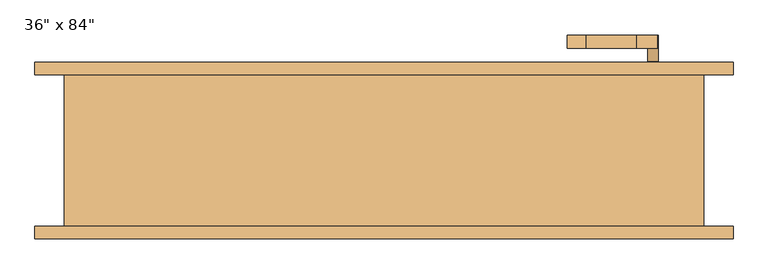
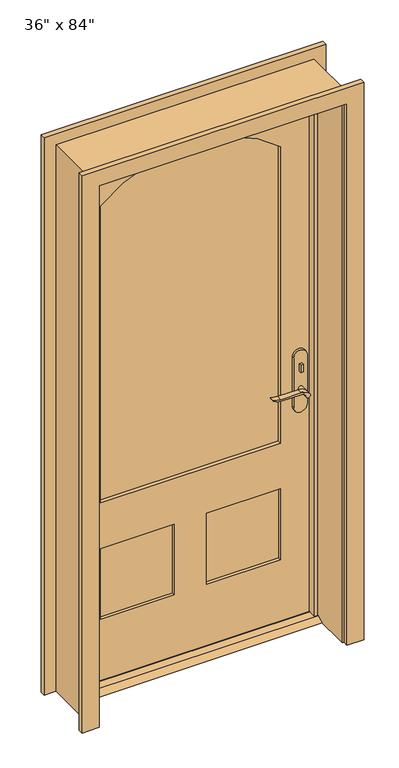
"""IFC4 building model written with IfcOpenShell, lengths in millimetres: door geometry."""

from ifc_helpers import new_model, si_unit, point, frame, frame_2d, origin, place, context, project, spatial, polyline, circle_curve, trimmed, segment, composite_curve, outline, extrude, faceted_brep, source, transform, mapped, element, save


def door_f079f64e(model_context):
    return source(origin(), model_context, "Body", "SolidModel", [
        extrude(outline(polyline([(38.1, 12.7), (73.025, 12.7), (98.425, 0.0), (12.7, 0.0), (38.1, 12.7)])), frame((-457.2, 0.0, 0.0), z_axis=(1.0, 0.0, 0.0), x_axis=(0.0, 1.0, 0.0)), (0.0, 0.0, 1.0), 914.4),
        extrude(outline(polyline([(411.4, 56.2), (401.4, 56.2), (401.4, 66.2), (411.4, 66.2), (411.4, 56.2)])), frame((0.0, 0.0, 981.9), z_axis=(0.0, 0.0, 1.0), x_axis=(1.0, 0.0, 0.0)), (0.0, 0.0, 1.0), 30.0),
        extrude(outline(composite_curve([segment(trimmed(circle_curve(frame_2d((996.9, 406.4)), 8.0), [point((996.9, 398.4))], [point((996.9, 414.4))], False, "CARTESIAN"), True, "CONTINUOUS"), segment(trimmed(circle_curve(frame_2d((996.9, 406.4)), 8.0), [point((996.9, 414.4))], [point((996.9, 398.4))], False, "CARTESIAN"), True, "CONTINUOUS")], self_intersect=False)), frame((0.0, 121.125, 0.0), z_axis=(0.0, 1.0, 0.0), x_axis=(0.0, 0.0, 1.0)), (0.0, 0.0, 1.0), 10.0),
        extrude(outline(composite_curve([segment(trimmed(circle_curve(frame_2d((897.1555521, 382.7324871)), 37.2832219), [point((919.0523287, 412.9081363))], [point((934.4, 381.0325667))], False, "CARTESIAN"), True, "CONTINUOUS"), segment(polyline([(934.4, 381.0325667), (934.4, 304.7564091)]), True, "CONTINUOUS"), segment(trimmed(circle_curve(frame_2d((1017.6850638, 304.8227909)), 83.2850902), [point((934.4, 304.7564091))], [point((939.4, 276.4))], True, "CARTESIAN"), True, "CONTINUOUS"), segment(polyline([(939.4, 276.4), (936.6135558, 276.4)]), True, "CONTINUOUS"), segment(trimmed(circle_curve(frame_2d((986.6709207, 308.3396612)), 59.3791355), [point((936.6135558, 276.4))], [point((927.4, 304.7564091))], False, "CARTESIAN"), True, "CONTINUOUS"), segment(polyline([(927.4, 304.7564091), (927.4, 381.0138099)]), True, "CONTINUOUS"), segment(trimmed(circle_curve(frame_2d((909.2738613, 381.0138099)), 18.1261387), [point((927.4, 381.0138099))], [point((914.4, 398.4))], True, "CARTESIAN"), True, "CONTINUOUS"), segment(trimmed(circle_curve(frame_2d((914.4, 406.4)), 8.0), [point((914.4, 398.4))], [point((919.0523287, 412.9081363))], False, "CARTESIAN"), True, "CONTINUOUS")], self_intersect=False)), frame((0.0, 16.2, 0.0), z_axis=(0.0, 1.0, 0.0), x_axis=(0.0, 0.0, 1.0)), (0.0, 0.0, 1.0), 20.0),
        extrude(outline(composite_curve([segment(trimmed(circle_curve(frame_2d((914.4, 406.4)), 8.0), [point((914.3999903, 398.4))], [point((919.0523287, 412.9081363))], False, "CARTESIAN"), True, "CONTINUOUS"), segment(trimmed(circle_curve(frame_2d((897.1555521, 382.7324871)), 37.2832219), [point((919.0523287, 412.9081363))], [point((934.4, 381.0325667))], False, "CARTESIAN"), True, "CONTINUOUS"), segment(polyline([(934.4, 381.0325667), (934.4, 304.7564091)]), True, "CONTINUOUS"), segment(trimmed(circle_curve(frame_2d((1017.6850638, 304.8227909)), 83.2850902), [point((934.4, 304.7564091))], [point((939.4, 276.4))], True, "CARTESIAN"), True, "CONTINUOUS"), segment(polyline([(939.4, 276.4), (936.6135558, 276.4)]), True, "CONTINUOUS"), segment(trimmed(circle_curve(frame_2d((986.6709207, 308.3396612)), 59.3791355), [point((936.6135558, 276.4))], [point((927.4, 304.7564091))], False, "CARTESIAN"), True, "CONTINUOUS"), segment(polyline([(927.4, 304.7564091), (927.4, 381.0138122)]), True, "CONTINUOUS"), segment(trimmed(circle_curve(frame_2d((909.2738682, 381.0138122)), 18.1261318), [point((927.4, 381.0138122))], [point((914.3999903, 398.4))], True, "CARTESIAN"), True, "CONTINUOUS")], self_intersect=False)), frame((0.0, 151.125, 0.0), z_axis=(0.0, 1.0, 0.0), x_axis=(0.0, 0.0, 1.0)), (0.0, 0.0, 1.0), 20.0),
        extrude(outline(composite_curve([segment(trimmed(circle_curve(frame_2d((914.4, 406.4)), 8.0), [point((914.4, 398.4))], [point((914.4, 414.4))], False, "CARTESIAN"), True, "CONTINUOUS"), segment(trimmed(circle_curve(frame_2d((914.4, 406.4)), 8.0), [point((914.4, 414.4))], [point((914.4, 398.4))], False, "CARTESIAN"), True, "CONTINUOUS")], self_intersect=False)), frame((0.0, 36.2, 0.0), z_axis=(0.0, 1.0, 0.0), x_axis=(0.0, 0.0, 1.0)), (0.0, 0.0, 1.0), 30.0),
        extrude(outline(composite_curve([segment(trimmed(circle_curve(frame_2d((914.4, 406.4)), 8.0), [point((914.4, 398.4))], [point((914.4, 414.4))], False, "CARTESIAN"), True, "CONTINUOUS"), segment(trimmed(circle_curve(frame_2d((914.4, 406.4)), 8.0), [point((914.4, 414.4))], [point((914.4, 398.4))], False, "CARTESIAN"), True, "CONTINUOUS")], self_intersect=False)), frame((0.0, 121.125, 0.0), z_axis=(0.0, 1.0, 0.0), x_axis=(0.0, 0.0, 1.0)), (0.0, 0.0, 1.0), 30.0),
        extrude(outline(composite_curve([segment(polyline([(844.4, 431.4), (1039.4, 431.4)]), True, "CONTINUOUS"), segment(trimmed(circle_curve(frame_2d((1039.4, 406.4)), 25.0), [point((1039.4, 431.4))], [point((1039.4, 381.4))], False, "CARTESIAN"), True, "CONTINUOUS"), segment(polyline([(1039.4, 381.4), (844.4, 381.4)]), True, "CONTINUOUS"), segment(trimmed(circle_curve(frame_2d((844.4, 406.4)), 25.0), [point((844.4, 381.4))], [point((844.4, 431.4))], False, "CARTESIAN"), True, "CONTINUOUS")], self_intersect=False)), frame((0.0, 66.2, 0.0), z_axis=(0.0, 1.0, 0.0), x_axis=(0.0, 0.0, 1.0)), (0.0, 0.0, 1.0), 10.0),
        extrude(outline(composite_curve([segment(polyline([(844.4, 431.4), (1039.4, 431.4)]), True, "CONTINUOUS"), segment(trimmed(circle_curve(frame_2d((1039.4, 406.4)), 25.0), [point((1039.4, 431.4))], [point((1039.4, 381.4))], False, "CARTESIAN"), True, "CONTINUOUS"), segment(polyline([(1039.4, 381.4), (844.4, 381.4)]), True, "CONTINUOUS"), segment(trimmed(circle_curve(frame_2d((844.4, 406.4)), 25.0), [point((844.4, 381.4))], [point((844.4, 431.4))], False, "CARTESIAN"), True, "CONTINUOUS")], self_intersect=False)), frame((0.0, 111.125, 0.0), z_axis=(0.0, 1.0, 0.0), x_axis=(0.0, 0.0, 1.0)), (0.0, 0.0, 1.0), 10.0),
        faceted_brep([(482.6, 111.125, 0.0), (482.6, -117.475, 0.0), (457.2, -117.475, 0.0), (457.2, 41.275, 0.0), (444.5, 41.275, 0.0), (444.5, 76.2, 0.0), (457.2, 76.2, 0.0), (457.2, 111.125, 0.0), (482.6, 111.125, 2159.0), (482.6, -117.475, 2159.0), (-482.6, -117.475, 2159.0), (-482.6, -117.475, 0.0), (-457.2, -117.475, 0.0), (-457.2, -117.475, 2133.6), (457.2, -117.475, 2133.6), (457.2, 41.275, 2133.6), (-457.2, 41.275, 2133.6), (-457.2, 41.275, 0.0), (-444.5, 41.275, 0.0), (-444.5, 41.275, 2120.9), (444.5, 41.275, 2120.9), (444.5, 76.2, 2120.9), (-444.5, 76.2, 2120.9), (-444.5, 76.2, 0.0), (-457.2, 76.2, 0.0), (-457.2, 76.2, 2133.6), (457.2, 76.2, 2133.6), (457.2, 111.125, 2133.6), (-457.2, 111.125, 2133.6), (-457.2, 111.125, 0.0), (-482.6, 111.125, 0.0), (-482.6, 111.125, 2159.0)], [[[0, 1, 2, 3, 4, 5, 6, 7]], [[1, 0, 8, 9]], [[2, 1, 9, 10, 11, 12, 13, 14]], [[3, 2, 14, 15]], [[4, 3, 15, 16, 17, 18, 19, 20]], [[5, 4, 20, 21]], [[6, 5, 21, 22, 23, 24, 25, 26]], [[7, 6, 26, 27]], [[0, 7, 27, 28, 29, 30, 31, 8]], [[9, 8, 31, 10]], [[15, 14, 13, 16]], [[21, 20, 19, 22]], [[27, 26, 25, 28]], [[30, 29, 24, 23, 18, 17, 12, 11]], [[10, 31, 30, 11]], [[16, 13, 12, 17]], [[22, 19, 18, 23]], [[28, 25, 24, 29]]]),
        extrude(outline(polyline([(2133.6, -457.2), (12.7, -457.2), (12.7, 457.2), (2133.6, 457.2), (2133.6, -457.2)]), holes=[composite_curve([segment(polyline([(714.375, -336.55), (1885.95, -336.55)]), True, "CONTINUOUS"), segment(trimmed(circle_curve(frame_2d((1503.52125, 0.0)), 509.42875), [point((1885.95, -336.55))], [point((1885.95, 336.55))], True, "CARTESIAN"), True, "CONTINUOUS"), segment(polyline([(1885.95, 336.55), (714.375, 336.55), (714.375, -336.55)]), True, "CONTINUOUS")], self_intersect=False), polyline([(533.4, -60.325), (254.0, -60.325), (254.0, -336.55), (533.4, -336.55), (533.4, -60.325)]), polyline([(533.4, 336.55), (254.0, 336.55), (254.0, 60.325), (533.4, 60.325), (533.4, 336.55)])]), frame((0.0, 76.2, 0.0), z_axis=(0.0, 1.0, 0.0), x_axis=(0.0, 0.0, 1.0)), (0.0, 0.0, 1.0), 34.925),
        extrude(outline(composite_curve([segment(polyline([(714.375, -336.55), (714.375, 336.55), (1885.95, 336.55)]), True, "CONTINUOUS"), segment(trimmed(circle_curve(frame_2d((1503.52125, 0.0)), 509.42875), [point((1885.95, 336.55))], [point((1885.95, -336.55))], False, "CARTESIAN"), True, "CONTINUOUS"), segment(polyline([(1885.95, -336.55), (714.375, -336.55)]), True, "CONTINUOUS")], self_intersect=False)), frame((0.0, 90.17, 0.0), z_axis=(0.0, 1.0, 0.0), x_axis=(0.0, 0.0, 1.0)), (0.0, 0.0, 1.0), 6.985),
        extrude(outline(polyline([(-60.325, 87.8416667), (-336.55, 87.8416667), (-336.55, 99.4833333), (-60.325, 99.4833333), (-60.325, 87.8416667)])), frame((0.0, 0.0, 254.0), z_axis=(0.0, 0.0, 1.0), x_axis=(1.0, 0.0, 0.0)), (0.0, 0.0, 1.0), 279.4),
        extrude(outline(polyline([(336.55, 87.8416667), (60.325, 87.8416667), (60.325, 99.4833333), (336.55, 99.4833333), (336.55, 87.8416667)])), frame((0.0, 0.0, 254.0), z_axis=(0.0, 0.0, 1.0), x_axis=(1.0, 0.0, 0.0)), (0.0, 0.0, 1.0), 279.4),
        extrude(outline(polyline([(0.0, -527.05), (0.0, -463.55), (2139.95, -463.55), (2139.95, 463.55), (0.0, 463.55), (0.0, 527.05), (2203.45, 527.05), (2203.45, -527.05), (0.0, -527.05)])), frame((0.0, 111.125, 0.0), z_axis=(0.0, 1.0, 0.0), x_axis=(0.0, 0.0, 1.0)), (0.0, 0.0, 1.0), 19.05),
        extrude(outline(polyline([(0.0, -527.05), (0.0, -463.55), (2139.95, -463.55), (2139.95, 463.55), (0.0, 463.55), (0.0, 527.05), (2203.45, 527.05), (2203.45, -527.05), (0.0, -527.05)])), frame((0.0, -136.525, 0.0), z_axis=(0.0, 1.0, 0.0), x_axis=(0.0, 0.0, 1.0)), (0.0, 0.0, 1.0), 19.05),
    ])


if __name__ == "__main__":
    model = new_model("IFC4")
    model_context = context("Model", 3, world=origin())
    ifc_project = project(units=[si_unit("LENGTHUNIT", "METRE", prefix="MILLI")], contexts=[model_context])
    site = spatial("IfcSite", under=ifc_project)
    building = spatial("IfcBuilding", under=site)
    placement = place(None, origin())
    door_shape = door_f079f64e(model_context)
    element("IfcDoor", 1, ObjectType="36\" x 84\"", at=placement, inside=building, context=model_context, shape_type="MappedRepresentation", body=[
        mapped(door_shape, transform((0.0, 0.0, 0.0), x_axis=(1.0, 0.0, 0.0), y_axis=(0.0, 1.0, 0.0), z_axis=(0.0, 0.0, 1.0))),
    ])
    save(model, "model.ifc")

# Revit data of these elements
# Type "36\" x 84\""
#   Type Mark = "11"
#   Assembly Code = "B2030100"
#   Analytic Construction = "French door, wood frame with single glass"
#   Threshold Offset [instance default] = 0' - 0 1/2"
#   Thickness = 0' - 1 3/8"
#   Thermal Resistance (R) = 1.0696 (h·ft²·°F)/BTU
#   Swing Angle [instance default] = 90.00°
#   Stiles = 0' - 4 3/4"
#   Rough Width = 3' - 2"
#   Rough Height = 7' - 1"
#   Radius = 1' - 8.05625"
#   Lock Rail = 0' - 7 1/8"
#   Height = 7' - 0"
#   Width = 3' - 0"
#   Heat Transfer Coefficient (U) = 0.9350 BTU/(h·ft²·°F)
#   Door Offset [instance default] = 0' - 0"
#   Bottom Rail = 0' - 9 1/2"
#   Threshold [instance default] = yes
#   Function = 1
#   Exterior Trim [instance default] = yes
#   Trim Material = Cherry
#   Threshold Material = Cherry
#   Panel Material = Cherry
#   Glazing = Glass
#   Frame Material = Cherry
#   Door Handle Material = Aluminum
#   Visual Light Transmittance = 0
#   Solar Heat Gain Coefficient = 0
#   Wall Closure = (empty or 0)
#   Construction Type = (empty or 0)
# Element 1 (IfcDoor, "36\" x 84\"")
#   Materials on its faces: "Cherry", "Aluminum", "Glass"
# Materials
#   "Cherry": class "Wood", colour RGB 226 177 128, transparency 0, Description = "Prunus Serotina", Cost = 0
#   "Glass": class "Glass", colour RGB 0 128 192, transparency 0.75, Description = "Soda Lime Glass", Cost = 0
#   "Aluminum": class "Metal", colour RGB 247 247 247, transparency 0, Description = "Aluminum 6061", Cost = 0
